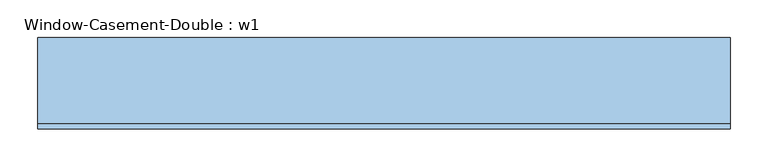
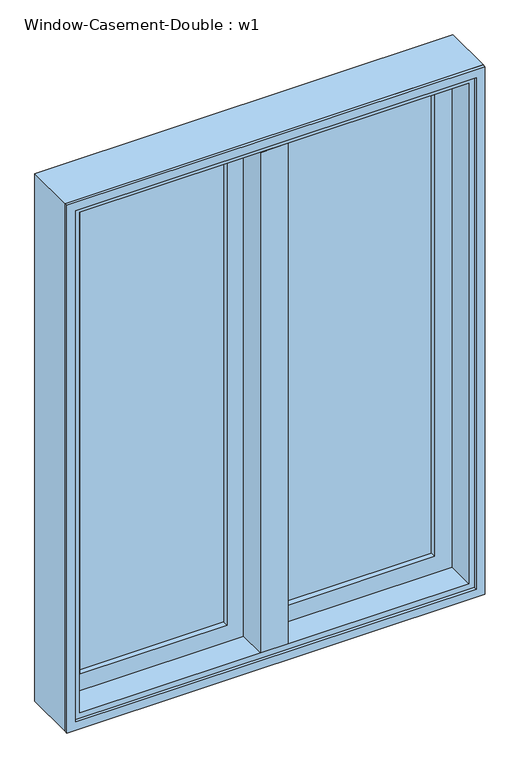
"""IFC4 building model written with IfcOpenShell, lengths in millimetres: window geometry, Window-Casement-Double : w1."""

from ifc_helpers import new_model, si_unit, frame, origin, place, context, project, spatial, polyline, outline, extrude, faceted_brep, source, transform, mapped, element, save


def window_casement_double_w1_80f1179f(model_context):
    return source(origin(), model_context, "Body", "SolidModel", [
        faceted_brep([(9.525, 69.85, 2120.9), (-9.525, 69.85, 2120.9), (-9.525, 19.05, 2120.9), (9.525, 19.05, 2120.9), (9.525, 69.85, 927.1), (9.525, 19.05, 927.1), (-9.525, 19.05, 927.1), (-9.525, 69.85, 927.1), (-9.525, 19.05, 946.15), (-9.525, 19.05, 2101.85), (-30.1625, 19.05, 946.15), (-30.1625, 19.05, 2101.85), (-30.1625, -44.45, 946.15), (-30.1625, -44.45, 2101.85), (30.1625, -44.45, 946.15), (30.1625, -44.45, 2101.85), (30.1625, 19.05, 946.15), (30.1625, 19.05, 2101.85), (9.525, 19.05, 946.15), (9.525, 19.05, 2101.85)], [[[0, 1, 2, 3]], [[4, 5, 6, 7]], [[1, 0, 4, 7]], [[2, 1, 7, 6, 8, 9]], [[9, 8, 10, 11]], [[11, 10, 12, 13]], [[13, 12, 14, 15]], [[15, 14, 16, 17]], [[17, 16, 18, 19]], [[0, 3, 19, 18, 5, 4]], [[18, 8, 6, 5]], [[9, 19, 3, 2]], [[8, 18, 16, 14, 12, 10]], [[19, 9, 11, 13, 15, 17]]]),
        extrude(outline(polyline([(-66.675, 50.8), (-66.675, 44.45), (-387.35, 44.45), (-387.35, 50.8), (-66.675, 50.8)])), frame((0.0, 0.0, 984.25), z_axis=(0.0, 0.0, 1.0), x_axis=(1.0, 0.0, 0.0)), (0.0, 0.0, 1.0), 1079.5),
        extrude(outline(polyline([(-387.35, 31.75), (-387.35, 38.1), (-66.675, 38.1), (-66.675, 31.75), (-387.35, 31.75)])), frame((0.0, 0.0, 984.25), z_axis=(0.0, 0.0, 1.0), x_axis=(1.0, 0.0, 0.0)), (0.0, 0.0, 1.0), 1079.5),
        extrude(outline(polyline([(387.35, 50.8), (387.35, 44.45), (66.675, 44.45), (66.675, 50.8), (387.35, 50.8)])), frame((0.0, 0.0, 984.25), z_axis=(0.0, 0.0, 1.0), x_axis=(1.0, 0.0, 0.0)), (0.0, 0.0, 1.0), 1079.5),
        extrude(outline(polyline([(66.675, 31.75), (66.675, 38.1), (387.35, 38.1), (387.35, 31.75), (66.675, 31.75)])), frame((0.0, 0.0, 984.25), z_axis=(0.0, 0.0, 1.0), x_axis=(1.0, 0.0, 0.0)), (0.0, 0.0, 1.0), 1079.5),
        extrude(outline(polyline([(2120.9, -444.5), (927.1, -444.5), (927.1, -9.525), (2120.9, -9.525), (2120.9, -444.5)]), holes=[polyline([(2063.75, -66.675), (984.25, -66.675), (984.25, -387.35), (2063.75, -387.35), (2063.75, -66.675)])]), frame((0.0, 19.05, 0.0), z_axis=(0.0, 1.0, 0.0), x_axis=(0.0, 0.0, 1.0)), (0.0, 0.0, 1.0), 44.45),
        extrude(outline(polyline([(927.1, 444.5), (2120.9, 444.5), (2120.9, 9.525), (927.1, 9.525), (927.1, 444.5)]), holes=[polyline([(984.25, 66.675), (2063.75, 66.675), (2063.75, 387.35), (984.25, 387.35), (984.25, 66.675)])]), frame((0.0, 19.05, 0.0), z_axis=(0.0, 1.0, 0.0), x_axis=(0.0, 0.0, 1.0)), (0.0, 0.0, 1.0), 44.45),
        extrude(outline(polyline([(2133.6, -457.2), (914.4, -457.2), (914.4, 457.2), (2133.6, 457.2), (2133.6, -457.2)]), holes=[polyline([(2114.55, 438.15), (933.45, 438.15), (933.45, -438.15), (2114.55, -438.15), (2114.55, 438.15)])]), frame((0.0, -50.8, 0.0), z_axis=(0.0, 1.0, 0.0), x_axis=(0.0, 0.0, 1.0)), (0.0, 0.0, 1.0), 6.35),
        faceted_brep([(425.45, 19.05, 2101.85), (425.45, -44.45, 2101.85), (-425.45, -44.45, 2101.85), (-425.45, 19.05, 2101.85), (444.5, 69.85, 2120.9), (444.5, 19.05, 2120.9), (-444.5, 19.05, 2120.9), (-444.5, 69.85, 2120.9), (457.2, -44.45, 2133.6), (457.2, 69.85, 2133.6), (-457.2, 69.85, 2133.6), (-457.2, -44.45, 2133.6), (-425.45, -44.45, 946.15), (-425.45, 19.05, 946.15), (-444.5, 19.05, 927.1), (-444.5, 69.85, 927.1), (-457.2, 69.85, 914.4), (-457.2, -44.45, 914.4), (425.45, -44.45, 946.15), (425.45, 19.05, 946.15), (444.5, 19.05, 927.1), (444.5, 69.85, 927.1), (457.2, 69.85, 914.4), (457.2, -44.45, 914.4)], [[[0, 1, 2, 3]], [[4, 5, 6, 7]], [[8, 9, 10, 11]], [[3, 2, 12, 13]], [[7, 6, 14, 15]], [[11, 10, 16, 17]], [[13, 12, 18, 19]], [[15, 14, 20, 21]], [[17, 16, 22, 23]], [[11, 17, 23, 8], [1, 18, 12, 2]], [[19, 18, 1, 0]], [[5, 20, 14, 6], [3, 13, 19, 0]], [[21, 20, 5, 4]], [[23, 22, 9, 8]], [[9, 22, 16, 10], [7, 15, 21, 4]]]),
    ])


if __name__ == "__main__":
    model = new_model("IFC4")
    model_context = context("Model", 3, world=origin())
    ifc_project = project(units=[si_unit("LENGTHUNIT", "METRE", prefix="MILLI")], contexts=[model_context])
    site = spatial("IfcSite", under=ifc_project)
    building = spatial("IfcBuilding", under=site)
    placement = place(None, origin())
    window_casement_double_w1_shape = window_casement_double_w1_80f1179f(model_context)
    element("IfcWindow", 1, ObjectType="Window-Casement-Double : w1", at=placement, inside=building, context=model_context, shape_type="MappedRepresentation", body=[
        mapped(window_casement_double_w1_shape, transform((0.0, 0.0, 0.0), x_axis=(1.0, 0.0, 0.0), y_axis=(0.0, 1.0, 0.0), z_axis=(0.0, 0.0, 1.0))),
    ])
    save(model, "model.ifc")

# Revit data of these elements
# Type "Window-Casement-Double : w1"
#   Type Mark = "14"
#   Fire Rating = "0.5h"
#   Assembly Code = "B2020100"
#   Analytic Construction = "Double glazing - domestic"
#   Frame Extension [instance default] = 0' - 0 1/4"
#   Window Inset [instance default] = 0' - 0"
#   Wall Thickness [instance default] = 0' - 6"
#   Interior Wall Closure [instance default] = 0' - 2 1/4"
#   Half Width = 1' - 6"
#   Visual Light Transmittance = 0.81
#   Thermal Resistance (R) = 1.8146 (h·ft²·°F)/BTU
#   Solar Heat Gain Coefficient = 0.76
#   Rough Width = 3' - 0 1/2"
#   Rough Height = 4' - 0 1/2"
#   Height = 4' - 0"
#   Heat Transfer Coefficient (U) = 0.5511 BTU/(h·ft²·°F)
#   Exterior Wall Closure [instance default] = 0' - 1 1/4"
#   Extension Jamb [instance default] = 0' - 2 1/4"
#   Default Sill Height = 3' - 0"
#   Width = 3' - 0"
#   Define Thermal Properties by = 0
#   Muntin Visibility = yes
#   Interior Trim Visibility [instance default] = yes
#   Exterior Trim Visibility [instance default] = yes
#   Extension Jamb Visibility [instance default] = yes
#   Muntin Pattern = Muntin Pattern_2x2 : Muntin Pattern_2x2
#   Interior Trim = Trim-Window-Interior-Flat : Picture Frame
#   Interior Frame Material = Wood - Stained
#   Glass Panel Material = Glass
#   Exterior Trim = Trim-Window-Exterior-Flat : with Sill
#   Wall Closure = (empty or 0)
# Element 1 (IfcWindow, "Window-Casement-Double : w1")
#   Wall Thickness = 0' - 4"
#   Extension Jamb = 0' - 0 1/4"
#   Materials on its faces: "Wood - Stained", "Glass"
# Materials
#   "Wood - Stained": class "Wood", colour RGB 224 178 126, transparency 0, Cost = 0
#   "Glass": class "Glass", colour RGB 0 128 192, transparency 0.75, Description = "Soda Lime Glass", Cost = 0
